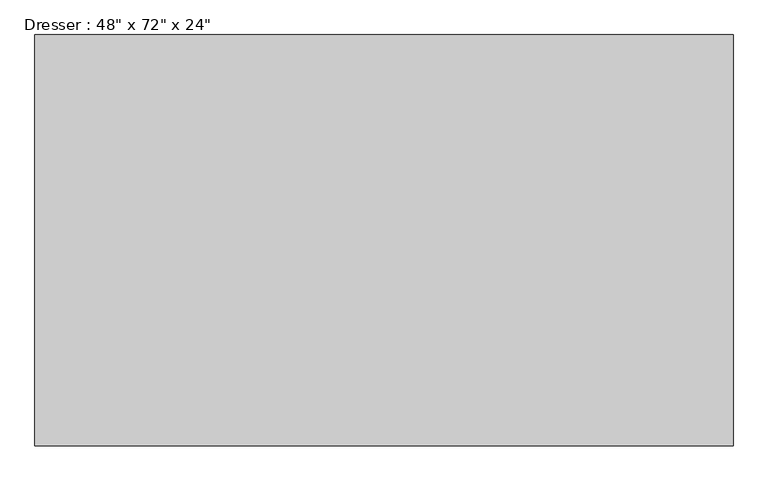
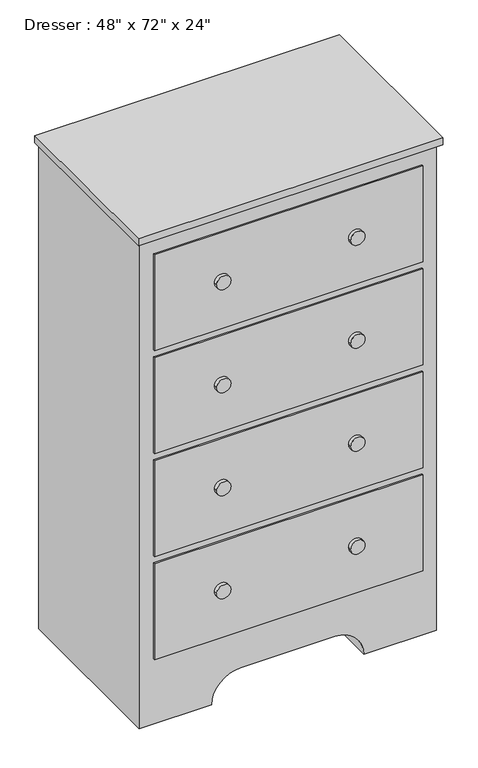
"""IFC4 building model written with IfcOpenShell, lengths in millimetres: furniture geometry."""

from ifc_helpers import new_model, si_unit, point, frame, frame_2d, origin, place, context, project, spatial, polyline, circle_curve, trimmed, segment, composite_curve, outline, extrude, source, transform, mapped, element, save


def furniture_f72bdee3(model_context):
    return source(origin(), model_context, "Body", "SweptSolid", [
        extrude(outline(polyline([(264.2067402, -58.3629541), (264.2067402, -687.0129541), (-802.5932598, -687.0129541), (-802.5932598, -58.3629541), (264.2067402, -58.3629541)])), frame((0.0, 0.0, 1803.4), z_axis=(0.0, 0.0, 1.0), x_axis=(1.0, 0.0, 0.0)), (0.0, 0.0, 1.0), 25.4),
        extrude(outline(composite_curve([segment(polyline([(0.0, 251.5067402), (1803.4, 251.5067402), (1803.4, -789.8932598), (0.0, -789.8932598), (0.0, -535.8932598)]), True, "CONTINUOUS"), segment(trimmed(circle_curve(frame_2d((0.0, -434.2932598)), 101.6), [point((0.0, -535.8932598))], [point((101.6, -434.2932598))], True, "CARTESIAN"), True, "CONTINUOUS"), segment(polyline([(101.6, -434.2932598), (101.6, -104.0932598)]), True, "CONTINUOUS"), segment(trimmed(circle_curve(frame_2d((0.0, -104.0932598)), 101.6), [point((101.6, -104.0932598))], [point((0.0, -2.4932598))], True, "CARTESIAN"), True, "CONTINUOUS"), segment(polyline([(0.0, -2.4932598), (0.0, 251.5067402)]), True, "CONTINUOUS")], self_intersect=False)), frame((0.0, -667.9629541, 0.0), z_axis=(0.0, 1.0, 0.0), x_axis=(0.0, 0.0, 1.0)), (0.0, 0.0, 1.0), 609.6),
        extrude(outline(composite_curve([segment(trimmed(circle_curve(frame_2d((1562.1, -34.2432598)), 25.4), [point((1562.1, -59.6432598))], [point((1562.1, -8.8432598))], False, "CARTESIAN"), True, "CONTINUOUS"), segment(trimmed(circle_curve(frame_2d((1562.1, -34.2432598)), 25.4), [point((1562.1, -8.8432598))], [point((1562.1, -59.6432598))], False, "CARTESIAN"), True, "CONTINUOUS")], self_intersect=False)), frame((0.0, -687.0129541, 0.0), z_axis=(0.0, 1.0, 0.0), x_axis=(0.0, 0.0, 1.0)), (0.0, 0.0, 1.0), 12.7),
        extrude(outline(composite_curve([segment(trimmed(circle_curve(frame_2d((1181.1, -34.2432598)), 25.4), [point((1181.1, -59.6432598))], [point((1181.1, -8.8432598))], False, "CARTESIAN"), True, "CONTINUOUS"), segment(trimmed(circle_curve(frame_2d((1181.1, -34.2432598)), 25.4), [point((1181.1, -8.8432598))], [point((1181.1, -59.6432598))], False, "CARTESIAN"), True, "CONTINUOUS")], self_intersect=False)), frame((0.0, -687.0129541, 0.0), z_axis=(0.0, 1.0, 0.0), x_axis=(0.0, 0.0, 1.0)), (0.0, 0.0, 1.0), 12.7),
        extrude(outline(composite_curve([segment(trimmed(circle_curve(frame_2d((800.1, -34.2432598)), 25.4), [point((800.1, -59.6432598))], [point((800.1, -8.8432598))], False, "CARTESIAN"), True, "CONTINUOUS"), segment(trimmed(circle_curve(frame_2d((800.1, -34.2432598)), 25.4), [point((800.1, -8.8432598))], [point((800.1, -59.6432598))], False, "CARTESIAN"), True, "CONTINUOUS")], self_intersect=False)), frame((0.0, -687.0129541, 0.0), z_axis=(0.0, 1.0, 0.0), x_axis=(0.0, 0.0, 1.0)), (0.0, 0.0, 1.0), 12.7),
        extrude(outline(composite_curve([segment(trimmed(circle_curve(frame_2d((419.1, -34.2432598)), 25.4), [point((419.1, -59.6432598))], [point((419.1, -8.8432598))], False, "CARTESIAN"), True, "CONTINUOUS"), segment(trimmed(circle_curve(frame_2d((419.1, -34.2432598)), 25.4), [point((419.1, -8.8432598))], [point((419.1, -59.6432598))], False, "CARTESIAN"), True, "CONTINUOUS")], self_intersect=False)), frame((0.0, -687.0129541, 0.0), z_axis=(0.0, 1.0, 0.0), x_axis=(0.0, 0.0, 1.0)), (0.0, 0.0, 1.0), 12.7),
        extrude(outline(composite_curve([segment(trimmed(circle_curve(frame_2d((419.1, -504.1432598)), 25.4), [point((419.1, -529.5432598))], [point((419.1, -478.7432598))], False, "CARTESIAN"), True, "CONTINUOUS"), segment(trimmed(circle_curve(frame_2d((419.1, -504.1432598)), 25.4), [point((419.1, -478.7432598))], [point((419.1, -529.5432598))], False, "CARTESIAN"), True, "CONTINUOUS")], self_intersect=False)), frame((0.0, -687.0129541, 0.0), z_axis=(0.0, 1.0, 0.0), x_axis=(0.0, 0.0, 1.0)), (0.0, 0.0, 1.0), 12.7),
        extrude(outline(composite_curve([segment(trimmed(circle_curve(frame_2d((800.1, -504.1432598)), 25.4), [point((800.1, -529.5432598))], [point((800.1, -478.7432598))], False, "CARTESIAN"), True, "CONTINUOUS"), segment(trimmed(circle_curve(frame_2d((800.1, -504.1432598)), 25.4), [point((800.1, -478.7432598))], [point((800.1, -529.5432598))], False, "CARTESIAN"), True, "CONTINUOUS")], self_intersect=False)), frame((0.0, -687.0129541, 0.0), z_axis=(0.0, 1.0, 0.0), x_axis=(0.0, 0.0, 1.0)), (0.0, 0.0, 1.0), 12.7),
        extrude(outline(composite_curve([segment(trimmed(circle_curve(frame_2d((1181.1, -504.1432598)), 25.4), [point((1181.1, -529.5432598))], [point((1181.1, -478.7432598))], False, "CARTESIAN"), True, "CONTINUOUS"), segment(trimmed(circle_curve(frame_2d((1181.1, -504.1432598)), 25.4), [point((1181.1, -478.7432598))], [point((1181.1, -529.5432598))], False, "CARTESIAN"), True, "CONTINUOUS")], self_intersect=False)), frame((0.0, -687.0129541, 0.0), z_axis=(0.0, 1.0, 0.0), x_axis=(0.0, 0.0, 1.0)), (0.0, 0.0, 1.0), 12.7),
        extrude(outline(composite_curve([segment(trimmed(circle_curve(frame_2d((1562.1, -504.1432598)), 25.4), [point((1562.1, -529.5432598))], [point((1562.1, -478.7432598))], False, "CARTESIAN"), True, "CONTINUOUS"), segment(trimmed(circle_curve(frame_2d((1562.1, -504.1432598)), 25.4), [point((1562.1, -478.7432598))], [point((1562.1, -529.5432598))], False, "CARTESIAN"), True, "CONTINUOUS")], self_intersect=False)), frame((0.0, -687.0129541, 0.0), z_axis=(0.0, 1.0, 0.0), x_axis=(0.0, 0.0, 1.0)), (0.0, 0.0, 1.0), 12.7),
        extrude(outline(polyline([(200.7067402, -674.3129541), (-739.0932598, -674.3129541), (-739.0932598, -667.9629541), (200.7067402, -667.9629541), (200.7067402, -674.3129541)])), frame((0.0, 0.0, 1384.3), z_axis=(0.0, 0.0, 1.0), x_axis=(1.0, 0.0, 0.0)), (0.0, 0.0, 1.0), 355.6),
        extrude(outline(polyline([(200.7067402, -674.3129541), (-739.0932598, -674.3129541), (-739.0932598, -667.9629541), (200.7067402, -667.9629541), (200.7067402, -674.3129541)])), frame((0.0, 0.0, 1003.3), z_axis=(0.0, 0.0, 1.0), x_axis=(1.0, 0.0, 0.0)), (0.0, 0.0, 1.0), 355.6),
        extrude(outline(polyline([(200.7067402, -674.3129541), (-739.0932598, -674.3129541), (-739.0932598, -667.9629541), (200.7067402, -667.9629541), (200.7067402, -674.3129541)])), frame((0.0, 0.0, 622.3), z_axis=(0.0, 0.0, 1.0), x_axis=(1.0, 0.0, 0.0)), (0.0, 0.0, 1.0), 355.6),
        extrude(outline(polyline([(200.7067402, -674.3129541), (-739.0932598, -674.3129541), (-739.0932598, -667.9629541), (200.7067402, -667.9629541), (200.7067402, -674.3129541)])), frame((0.0, 0.0, 241.3), z_axis=(0.0, 0.0, 1.0), x_axis=(1.0, 0.0, 0.0)), (0.0, 0.0, 1.0), 355.6),
    ])


if __name__ == "__main__":
    model = new_model("IFC4")
    model_context = context("Model", 3, world=origin())
    ifc_project = project(units=[si_unit("LENGTHUNIT", "METRE", prefix="MILLI")], contexts=[model_context])
    site = spatial("IfcSite", under=ifc_project)
    building = spatial("IfcBuilding", under=site)
    placement = place(None, origin())
    furniture_shape = furniture_f72bdee3(model_context)
    element("IfcFurniture", 1, ObjectType="Dresser : 48\" x 72\" x 24\"", at=placement, inside=building, context=model_context, shape_type="MappedRepresentation", body=[
        mapped(furniture_shape, transform((0.0, 0.0, 0.0), x_axis=(1.0, 0.0, 0.0), y_axis=(0.0, 1.0, 0.0), z_axis=(0.0, 0.0, 1.0))),
    ])
    save(model, "model.ifc")

# Revit data of these elements
# Type "Dresser : 48\" x 72\" x 24\""
#   Assembly Code = "E2020200"
#   Depth = 2' - 0"
#   Height = 6' - 0"
#   Width = 3' - 5"
#   Dresser Material = Wood
#   Drawer Material = Wood
#   Knob Material = Cherry
#   Default Elevation = 0
# Element 1 (IfcFurniture, "Dresser : 48\" x 72\" x 24\"")
#   Materials on its faces: "Laminate, Ivory, Matte", "Cherry", "Wood"
# Materials
#   "Wood": class "Wood", colour RGB 0 0 0, transparency 0, Description = "Generic wood", Cost = 0
#   "Cherry": class "Wood", colour RGB 226 177 128, transparency 0, Description = "Prunus Serotina", Cost = 0
#   "Laminate, Ivory, Matte": class "Plastic", colour RGB 247 247 239, transparency 0, Description = "Plastic Laminate - Ivory, Matte", Cost = 0
